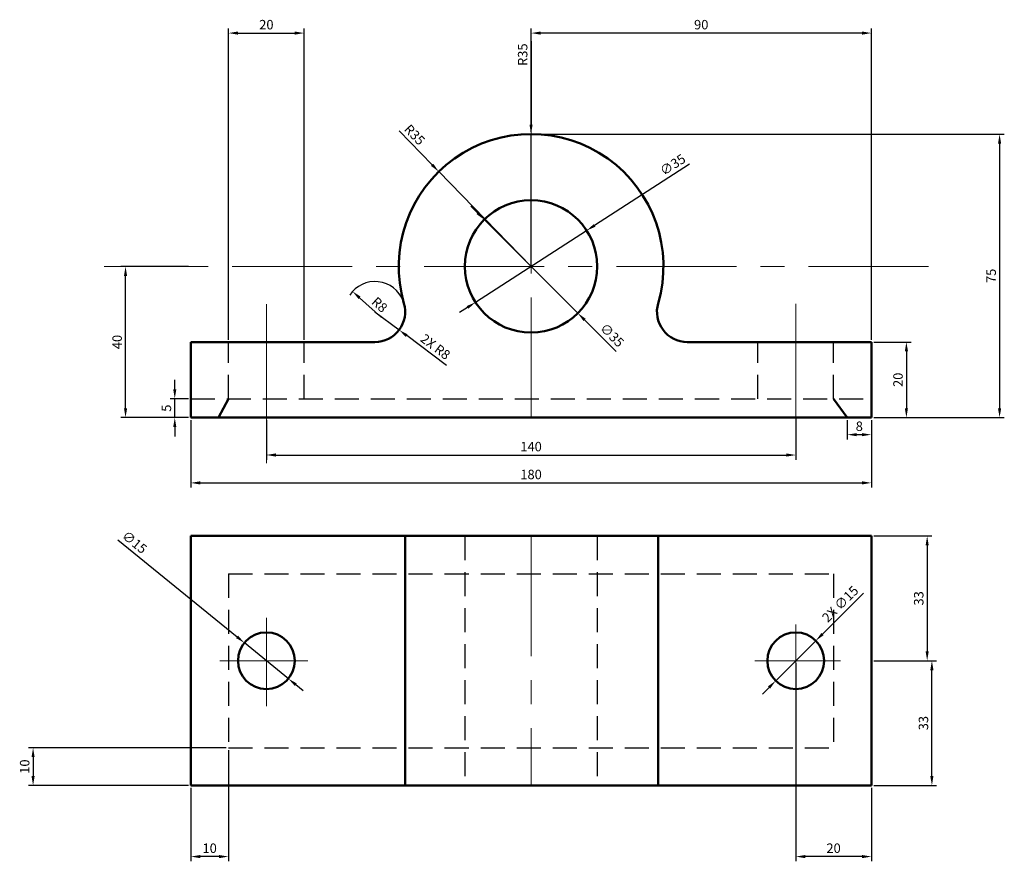
# Model space of a CAD drawing. Units: millimetres. Extents: x 2529 to 2789, y 1399 to 1622.
import ezdxf

# ---------------------------------------------------------------- set-up
doc = ezdxf.new("R2010")
doc.units = ezdxf.units.MM
doc.linetypes.add('CENTER', pattern=[50.8, 31.75, -6.35, 6.35, -6.35])
doc.linetypes.add('HIDDEN', pattern=[9.525, 6.35, -3.175])
for name, color, linetype, lineweight in [('M-CNTR', 1, 'CENTER', 18), ('M-DIMS', 2, 'Continuous', 25), ('M-HIDN', 4, 'HIDDEN', 25), ('M-OUTL', 7, 'Continuous', 50)]:
    doc.layers.add(name, color=color, linetype=linetype, lineweight=lineweight)
doc.styles.get("Standard").update_dxf_attribs({"font": 'arial.ttf'})
doc.dimstyles.new('ISO-25', dxfattribs={"dimtxt": 2.5, "dimasz": 2.5, "dimexe": 1.25, "dimexo": 0.625, "dimtad": 1, "dimtxsty": 'Standard', "dimcen": 2.5, "dimadec": 0, "dimazin": 0, "dimtfac": 1, "dimtmove": 0, "dimatfit": 3, "dimfxl": 1, "dimarcsym": 0})

# ---------------------------------------------------------------- blocks, each defined once
blk = doc.blocks.new('*D1')
at = {"layer": 'Defpoints', "color": 0, "transparency": 16777216}
for p in [(2747.84, 1516.67), (2754.23, 1516.67), (2747.84, 1512.16)]:
    blk.add_point(p, dxfattribs=at)
at = {"layer": 'M-DIMS', "color": 0, "lineweight": -2, "transparency": 16777216}
for p, q in [((2747.84, 1516.04), (2747.84, 1510.91)), ((2754.23, 1516.04), (2754.23, 1510.91)), ((2751.73, 1512.16), (2750.34, 1512.16))]:
    blk.add_line(p, q, dxfattribs=at)
at = {"layer": 'M-DIMS', "color": 0, "transparency": 16777216}
for points in [[(2750.34, 1512.58), (2750.34, 1511.75), (2747.84, 1512.16)], [(2751.73, 1512.58), (2751.73, 1511.75), (2754.23, 1512.16)]]:
    blk.add_solid(points, dxfattribs=at)
at = {"layer": 'M-DIMS', "color": 0, "transparency": 16777216, "insert": (2751.03, 1514.06), "char_height": 2.5, "attachment_point": 5}
blk.add_mtext('8', dxfattribs=at)
blk = doc.blocks.new('*D2')
at = {"layer": 'Defpoints', "color": 0, "transparency": 16777216}
for p in [(2754.23, 1485.36), (2754.23, 1452.36), (2768.98, 1452.36)]:
    blk.add_point(p, dxfattribs=at)
at = {"layer": 'M-DIMS', "color": 0, "lineweight": -2, "transparency": 16777216}
for p, q in [((2754.85, 1485.36), (2770.23, 1485.36)), ((2768.98, 1482.86), (2768.98, 1454.86)), ((2754.85, 1452.36), (2770.23, 1452.36))]:
    blk.add_line(p, q, dxfattribs=at)
at = {"layer": 'M-DIMS', "color": 0, "transparency": 16777216}
for points in [[(2768.56, 1482.86), (2769.39, 1482.86), (2768.98, 1485.36)], [(2768.56, 1454.86), (2769.39, 1454.86), (2768.98, 1452.36)]]:
    blk.add_solid(points, dxfattribs=at)
at = {"layer": 'M-DIMS', "color": 0, "transparency": 16777216, "insert": (2767.07, 1468.86), "char_height": 2.5, "attachment_point": 5, "rotation": 90}
blk.add_mtext('33', dxfattribs=at)
blk = doc.blocks.new('*D3')
at = {"layer": 'Defpoints', "color": 0, "transparency": 16777216}
for p in [(2754.23, 1452.36), (2770.23, 1452.36), (2754.23, 1419.36)]:
    blk.add_point(p, dxfattribs=at)
at = {"layer": 'M-DIMS', "color": 0, "lineweight": -2, "transparency": 16777216}
for p, q in [((2754.85, 1452.36), (2771.48, 1452.36)), ((2770.23, 1421.86), (2770.23, 1449.86)), ((2754.85, 1419.36), (2771.48, 1419.36))]:
    blk.add_line(p, q, dxfattribs=at)
at = {"layer": 'M-DIMS', "color": 0, "transparency": 16777216}
for points in [[(2769.81, 1449.86), (2770.64, 1449.86), (2770.23, 1452.36)], [(2769.81, 1421.86), (2770.64, 1421.86), (2770.23, 1419.36)]]:
    blk.add_solid(points, dxfattribs=at)
at = {"layer": 'M-DIMS', "color": 0, "transparency": 16777216, "insert": (2768.32, 1435.86), "char_height": 2.5, "attachment_point": 5, "rotation": 90}
blk.add_mtext('33', dxfattribs=at)
blk = doc.blocks.new('*D4')
at = {"layer": 'Defpoints', "color": 0, "transparency": 16777216}
for p in [(2588.41, 1457.1), (2600.04, 1447.62)]:
    blk.add_point(p, dxfattribs=at)
at = {"layer": 'M-DIMS', "color": 0, "lineweight": -2, "transparency": 16777216}
for p, q in [((2554.98, 1484.33), (2586.48, 1458.68)), ((2600.04, 1447.62), (2588.41, 1457.1)), ((2601.98, 1446.04), (2603.92, 1444.46))]:
    blk.add_line(p, q, dxfattribs=at)
at = {"layer": 'M-DIMS', "color": 0, "transparency": 16777216}
for points in [[(2586.74, 1459), (2586.21, 1458.35), (2588.41, 1457.1)], [(2602.24, 1446.37), (2601.72, 1445.72), (2600.04, 1447.62)]]:
    blk.add_solid(points, dxfattribs=at)
at = {"layer": 'M-DIMS', "color": 0, "transparency": 16777216, "insert": (2559.16, 1483.47), "char_height": 2.5, "attachment_point": 5, "rotation": 320.8294}
blk.add_mtext('∅15', dxfattribs=at)
blk = doc.blocks.new('*D5')
at = {"layer": 'Defpoints', "color": 0, "transparency": 16777216}
for p in [(2574.23, 1516.67), (2754.23, 1516.67), (2754.23, 1499.41)]:
    blk.add_point(p, dxfattribs=at)
at = {"layer": 'M-DIMS', "color": 0, "lineweight": -2, "transparency": 16777216}
for p, q in [((2574.23, 1516.04), (2574.23, 1498.16)), ((2754.23, 1516.04), (2754.23, 1498.16)), ((2576.73, 1499.41), (2751.73, 1499.41))]:
    blk.add_line(p, q, dxfattribs=at)
at = {"layer": 'M-DIMS', "color": 0, "transparency": 16777216}
for points in [[(2576.73, 1499.83), (2576.73, 1498.99), (2574.23, 1499.41)], [(2751.73, 1499.83), (2751.73, 1498.99), (2754.23, 1499.41)]]:
    blk.add_solid(points, dxfattribs=at)
at = {"layer": 'M-DIMS', "color": 0, "transparency": 16777216, "insert": (2664.23, 1501.31), "char_height": 2.5, "attachment_point": 5}
blk.add_mtext('180', dxfattribs=at)
blk = doc.blocks.new('*D6')
at = {"layer": 'Defpoints', "color": 0, "transparency": 16777216}
for p in [(2594.23, 1516.67), (2734.23, 1517.07), (2734.23, 1506.78)]:
    blk.add_point(p, dxfattribs=at)
at = {"layer": 'M-DIMS', "color": 0, "lineweight": -2, "transparency": 16777216}
for p, q in [((2594.23, 1516.04), (2594.23, 1505.53)), ((2734.23, 1516.44), (2734.23, 1505.53)), ((2596.73, 1506.78), (2731.73, 1506.78))]:
    blk.add_line(p, q, dxfattribs=at)
at = {"layer": 'M-DIMS', "color": 0, "transparency": 16777216}
for points in [[(2596.73, 1507.2), (2596.73, 1506.36), (2594.23, 1506.78)], [(2731.73, 1507.2), (2731.73, 1506.36), (2734.23, 1506.78)]]:
    blk.add_solid(points, dxfattribs=at)
at = {"layer": 'M-DIMS', "color": 0, "transparency": 16777216, "insert": (2664.23, 1508.68), "char_height": 2.5, "attachment_point": 5}
blk.add_mtext('140', dxfattribs=at)
blk = doc.blocks.new('*D7')
at = {"layer": 'Defpoints', "color": 0, "transparency": 16777216}
for p in [(2570.01, 1521.67), (2574.23, 1521.67), (2574.23, 1516.67)]:
    blk.add_point(p, dxfattribs=at)
at = {"layer": 'M-DIMS', "color": 0, "lineweight": -2, "transparency": 16777216}
for p, q in [((2570.01, 1524.17), (2570.01, 1526.67)), ((2573.6, 1521.67), (2568.76, 1521.67)), ((2570.01, 1516.67), (2570.01, 1521.67)), ((2573.6, 1516.67), (2568.76, 1516.67)), ((2570.01, 1514.17), (2570.01, 1511.67))]:
    blk.add_line(p, q, dxfattribs=at)
at = {"layer": 'M-DIMS', "color": 0, "transparency": 16777216}
for points in [[(2569.59, 1524.17), (2570.42, 1524.17), (2570.01, 1521.67)], [(2569.59, 1514.17), (2570.42, 1514.17), (2570.01, 1516.67)]]:
    blk.add_solid(points, dxfattribs=at)
at = {"layer": 'M-DIMS', "color": 0, "transparency": 16777216, "insert": (2568.11, 1519.17), "char_height": 2.5, "attachment_point": 5, "rotation": 90}
blk.add_mtext('5', dxfattribs=at)
blk = doc.blocks.new('*D8')
at = {"layer": 'Defpoints', "color": 0, "transparency": 16777216}
for p in [(2556.98, 1556.67), (2574.23, 1556.67), (2574.23, 1516.67)]:
    blk.add_point(p, dxfattribs=at)
at = {"layer": 'M-DIMS', "color": 0, "lineweight": -2, "transparency": 16777216}
for p, q in [((2573.6, 1556.67), (2555.73, 1556.67)), ((2556.98, 1519.17), (2556.98, 1554.17)), ((2573.6, 1516.67), (2555.73, 1516.67))]:
    blk.add_line(p, q, dxfattribs=at)
at = {"layer": 'M-DIMS', "color": 0, "transparency": 16777216}
for points in [[(2556.57, 1554.17), (2557.4, 1554.17), (2556.98, 1556.67)], [(2556.57, 1519.17), (2557.4, 1519.17), (2556.98, 1516.67)]]:
    blk.add_solid(points, dxfattribs=at)
at = {"layer": 'M-DIMS', "color": 0, "transparency": 16777216, "insert": (2555.08, 1536.67), "char_height": 2.5, "attachment_point": 5, "rotation": 90}
blk.add_mtext('40', dxfattribs=at)
blk = doc.blocks.new('*D9')
at = {"layer": 'Defpoints', "color": 0, "transparency": 16777216}
for p in [(2617.02, 1550.05), (2622.94, 1544.67)]:
    blk.add_point(p, dxfattribs=at)
at = {"layer": 'M-DIMS', "color": 0, "lineweight": -2, "transparency": 16777216}
blk.add_line((2624.63, 1543.13), (2618.87, 1548.37), dxfattribs=at)
blk.add_arc((2622.94, 1544.67), 8, 20.6809, 146.6391, dxfattribs=at)
at = {"layer": 'M-DIMS', "color": 0, "transparency": 16777216}
blk.add_solid([(2619.15, 1548.68), (2618.59, 1548.06), (2617.02, 1550.05)], dxfattribs=at)
at = {"layer": 'M-DIMS', "color": 0, "transparency": 16777216, "insert": (2623.95, 1546.31), "char_height": 2.5, "attachment_point": 5, "rotation": 317.6867}
blk.add_mtext('R8', dxfattribs=at)
blk = doc.blocks.new('*D10')
at = {"layer": 'Defpoints', "color": 0, "transparency": 16777216}
for p in [(2754.23, 1536.67), (2754.23, 1516.67), (2763.49, 1516.67)]:
    blk.add_point(p, dxfattribs=at)
at = {"layer": 'M-DIMS', "color": 0, "lineweight": -2, "transparency": 16777216}
for p, q in [((2754.85, 1536.67), (2764.74, 1536.67)), ((2763.49, 1534.17), (2763.49, 1519.17)), ((2754.85, 1516.67), (2764.74, 1516.67))]:
    blk.add_line(p, q, dxfattribs=at)
at = {"layer": 'M-DIMS', "color": 0, "transparency": 16777216}
for points in [[(2763.07, 1534.17), (2763.91, 1534.17), (2763.49, 1536.67)], [(2763.07, 1519.17), (2763.91, 1519.17), (2763.49, 1516.67)]]:
    blk.add_solid(points, dxfattribs=at)
at = {"layer": 'M-DIMS', "color": 0, "transparency": 16777216, "insert": (2761.59, 1526.67), "char_height": 2.5, "attachment_point": 5, "rotation": 90}
blk.add_mtext('20', dxfattribs=at)
blk = doc.blocks.new('*D11')
at = {"layer": 'Defpoints', "color": 0, "transparency": 16777216}
for p in [(2678.93, 1566.16), (2649.52, 1547.18)]:
    blk.add_point(p, dxfattribs=at)
at = {"layer": 'M-DIMS', "color": 0, "lineweight": -2, "transparency": 16777216}
for p, q in [((2706.1, 1583.69), (2681.03, 1567.51)), ((2649.52, 1547.18), (2678.93, 1566.16)), ((2647.42, 1545.82), (2645.32, 1544.47))]:
    blk.add_line(p, q, dxfattribs=at)
at = {"layer": 'M-DIMS', "color": 0, "transparency": 16777216}
for points in [[(2680.81, 1567.86), (2681.26, 1567.16), (2678.93, 1566.16)], [(2647.2, 1546.17), (2647.65, 1545.47), (2649.52, 1547.18)]]:
    blk.add_solid(points, dxfattribs=at)
at = {"layer": 'M-DIMS', "color": 0, "transparency": 16777216, "insert": (2701.85, 1583.29), "char_height": 2.5, "attachment_point": 5, "rotation": 32.8304}
blk.add_mtext('∅35', dxfattribs=at)
blk = doc.blocks.new('*D12')
at = {"layer": 'Defpoints', "color": 0, "transparency": 16777216}
for p in [(2639.81, 1581.75), (2664.23, 1556.67)]:
    blk.add_point(p, dxfattribs=at)
at = {"layer": 'M-DIMS', "color": 0, "lineweight": -2, "transparency": 16777216}
for p, q in [((2629.31, 1592.54), (2638.07, 1583.54)), ((2664.23, 1556.67), (2639.81, 1581.75))]:
    blk.add_line(p, q, dxfattribs=at)
at = {"layer": 'M-DIMS', "color": 0, "transparency": 16777216}
blk.add_solid([(2638.37, 1583.83), (2637.77, 1583.25), (2639.81, 1581.75)], dxfattribs=at)
at = {"layer": 'M-DIMS', "color": 0, "transparency": 16777216, "insert": (2633.2, 1591.27), "char_height": 2.5, "attachment_point": 5, "rotation": 314.2295}
blk.add_mtext('R35', dxfattribs=at)
blk = doc.blocks.new('MOUNT-HOLE-D15')
blk.add_circle((7.5, 7.5), 7.5)
blk = doc.blocks.new('MOUNT-HOLE-ELEV')
for p, q in [((0, 0), (0, 15)), ((20, 0), (20, 15))]:
    blk.add_line(p, q)
blk = doc.blocks.new('*D15')
at = {"layer": 'Defpoints', "color": 0, "transparency": 16777216}
for p in [(2664.23, 1591.67), (2754.23, 1516.67), (2788.13, 1516.67)]:
    blk.add_point(p, dxfattribs=at)
at = {"layer": 'M-DIMS', "color": 0, "lineweight": -2, "transparency": 16777216}
for p, q in [((2664.85, 1591.67), (2789.38, 1591.67)), ((2788.13, 1589.17), (2788.13, 1519.17)), ((2754.85, 1516.67), (2789.38, 1516.67))]:
    blk.add_line(p, q, dxfattribs=at)
at = {"layer": 'M-DIMS', "color": 0, "transparency": 16777216}
for points in [[(2787.71, 1589.17), (2788.55, 1589.17), (2788.13, 1591.67)], [(2787.71, 1519.17), (2788.55, 1519.17), (2788.13, 1516.67)]]:
    blk.add_solid(points, dxfattribs=at)
at = {"layer": 'M-DIMS', "color": 0, "transparency": 16777216, "insert": (2786.23, 1554.17), "char_height": 2.5, "attachment_point": 5, "rotation": 90}
blk.add_mtext('75', dxfattribs=at)
blk = doc.blocks.new('*D16')
at = {"layer": 'Defpoints', "color": 0, "transparency": 16777216}
for p in [(2734.23, 1452.36), (2754.23, 1419.36), (2734.23, 1400.56)]:
    blk.add_point(p, dxfattribs=at)
at = {"layer": 'M-DIMS', "color": 0, "lineweight": -2, "transparency": 16777216}
for p, q in [((2734.23, 1451.73), (2734.23, 1399.31)), ((2754.23, 1418.73), (2754.23, 1399.31)), ((2751.73, 1400.56), (2736.73, 1400.56))]:
    blk.add_line(p, q, dxfattribs=at)
at = {"layer": 'M-DIMS', "color": 0, "transparency": 16777216}
for points in [[(2736.73, 1400.98), (2736.73, 1400.14), (2734.23, 1400.56)], [(2751.73, 1400.98), (2751.73, 1400.14), (2754.23, 1400.56)]]:
    blk.add_solid(points, dxfattribs=at)
at = {"layer": 'M-DIMS', "color": 0, "transparency": 16777216, "insert": (2744.23, 1402.46), "char_height": 2.5, "attachment_point": 5}
blk.add_mtext('20', dxfattribs=at)
blk = doc.blocks.new('*D17')
at = {"layer": 'Defpoints', "color": 0, "transparency": 16777216}
for p in [(2664.23, 1618.39), (2664.23, 1591.67), (2754.23, 1536.67)]:
    blk.add_point(p, dxfattribs=at)
at = {"layer": 'M-DIMS', "color": 0, "lineweight": -2, "transparency": 16777216}
for p, q in [((2664.23, 1592.29), (2664.23, 1619.64)), ((2754.23, 1537.29), (2754.23, 1619.64)), ((2751.73, 1618.39), (2666.73, 1618.39))]:
    blk.add_line(p, q, dxfattribs=at)
at = {"layer": 'M-DIMS', "color": 0, "transparency": 16777216}
for points in [[(2666.73, 1618.8), (2666.73, 1617.97), (2664.23, 1618.39)], [(2751.73, 1618.8), (2751.73, 1617.97), (2754.23, 1618.39)]]:
    blk.add_solid(points, dxfattribs=at)
at = {"layer": 'M-DIMS', "color": 0, "transparency": 16777216, "insert": (2709.23, 1620.29), "char_height": 2.5, "attachment_point": 5}
blk.add_mtext('90', dxfattribs=at)
blk = doc.blocks.new('*D18')
at = {"layer": 'Defpoints', "color": 0, "transparency": 16777216}
for p in [(2584.23, 1429.36), (2532.53, 1419.36), (2574.23, 1419.36)]:
    blk.add_point(p, dxfattribs=at)
at = {"layer": 'M-DIMS', "color": 0, "lineweight": -2, "transparency": 16777216}
for p, q in [((2583.6, 1429.36), (2531.28, 1429.36)), ((2532.53, 1426.86), (2532.53, 1421.86)), ((2573.6, 1419.36), (2531.28, 1419.36))]:
    blk.add_line(p, q, dxfattribs=at)
at = {"layer": 'M-DIMS', "color": 0, "transparency": 16777216}
for points in [[(2532.12, 1426.86), (2532.95, 1426.86), (2532.53, 1429.36)], [(2532.12, 1421.86), (2532.95, 1421.86), (2532.53, 1419.36)]]:
    blk.add_solid(points, dxfattribs=at)
at = {"layer": 'M-DIMS', "color": 0, "transparency": 16777216, "insert": (2530.63, 1424.36), "char_height": 2.5, "attachment_point": 5, "rotation": 90}
blk.add_mtext('10', dxfattribs=at)
blk = doc.blocks.new('*D19')
at = {"layer": 'Defpoints', "color": 0, "transparency": 16777216}
for p in [(2584.23, 1429.36), (2574.23, 1419.36), (2574.23, 1400.56)]:
    blk.add_point(p, dxfattribs=at)
at = {"layer": 'M-DIMS', "color": 0, "lineweight": -2, "transparency": 16777216}
for p, q in [((2584.23, 1428.73), (2584.23, 1399.31)), ((2574.23, 1418.73), (2574.23, 1399.31)), ((2581.73, 1400.56), (2576.73, 1400.56))]:
    blk.add_line(p, q, dxfattribs=at)
at = {"layer": 'M-DIMS', "color": 0, "transparency": 16777216}
for points in [[(2576.73, 1400.98), (2576.73, 1400.14), (2574.23, 1400.56)], [(2581.73, 1400.98), (2581.73, 1400.14), (2584.23, 1400.56)]]:
    blk.add_solid(points, dxfattribs=at)
at = {"layer": 'M-DIMS', "color": 0, "transparency": 16777216, "insert": (2579.23, 1402.46), "char_height": 2.5, "attachment_point": 5}
blk.add_mtext('10', dxfattribs=at)
blk = doc.blocks.new('*D20')
at = {"layer": 'Defpoints', "color": 0, "transparency": 16777216}
for p in [(2604.23, 1618.39), (2584.23, 1536.67), (2604.23, 1536.67)]:
    blk.add_point(p, dxfattribs=at)
at = {"layer": 'M-DIMS', "color": 0, "lineweight": -2, "transparency": 16777216}
for p, q in [((2584.23, 1537.29), (2584.23, 1619.64)), ((2604.23, 1537.29), (2604.23, 1619.64)), ((2586.73, 1618.39), (2601.73, 1618.39))]:
    blk.add_line(p, q, dxfattribs=at)
at = {"layer": 'M-DIMS', "color": 0, "transparency": 16777216}
for points in [[(2586.73, 1618.8), (2586.73, 1617.97), (2584.23, 1618.39)], [(2601.73, 1618.8), (2601.73, 1617.97), (2604.23, 1618.39)]]:
    blk.add_solid(points, dxfattribs=at)
at = {"layer": 'M-DIMS', "color": 0, "transparency": 16777216, "insert": (2594.23, 1620.29), "char_height": 2.5, "attachment_point": 5}
blk.add_mtext('20', dxfattribs=at)
blk = doc.blocks.new('*D21')
at = {"layer": 'Defpoints', "color": 0, "transparency": 16777216}
for p in [(2664.23, 1591.67), (2664.23, 1556.67)]:
    blk.add_point(p, dxfattribs=at)
at = {"layer": 'M-DIMS', "color": 0, "lineweight": -2, "transparency": 16777216}
for p, q in [((2664.23, 1616.29), (2664.23, 1594.17)), ((2664.23, 1556.67), (2664.23, 1591.67))]:
    blk.add_line(p, q, dxfattribs=at)
at = {"layer": 'M-DIMS', "color": 0, "transparency": 16777216}
blk.add_solid([(2663.81, 1594.17), (2664.64, 1594.17), (2664.23, 1591.67)], dxfattribs=at)
at = {"layer": 'M-DIMS', "color": 0, "transparency": 16777216, "insert": (2662.33, 1612.67), "char_height": 2.5, "attachment_point": 5, "rotation": 89.9999}
blk.add_mtext('R35', dxfattribs=at)
blk = doc.blocks.new('*D22')
at = {"layer": 'Defpoints', "color": 0, "transparency": 16777216}
for p in [(2651.85, 1569.04), (2676.6, 1544.29)]:
    blk.add_point(p, dxfattribs=at)
at = {"layer": 'M-DIMS', "color": 0, "lineweight": -2, "transparency": 16777216}
for p, q in [((2650.09, 1570.81), (2648.32, 1572.58)), ((2651.85, 1569.04), (2676.6, 1544.29)), ((2686.7, 1534.19), (2678.37, 1542.53))]:
    blk.add_line(p, q, dxfattribs=at)
at = {"layer": 'M-DIMS', "color": 0, "transparency": 16777216}
for points in [[(2650.38, 1571.1), (2649.79, 1570.51), (2651.85, 1569.04)], [(2678.66, 1542.82), (2678.08, 1542.23), (2676.6, 1544.29)]]:
    blk.add_solid(points, dxfattribs=at)
at = {"layer": 'M-DIMS', "color": 0, "transparency": 16777216, "insert": (2685.42, 1538.26), "char_height": 2.5, "attachment_point": 5, "rotation": 315.0011}
blk.add_mtext('∅35', dxfattribs=at)
blk = doc.blocks.new('*D23')
at = {"layer": 'Defpoints', "color": 0, "transparency": 16777216}
for p in [(2622.94, 1544.67), (2629.33, 1539.86)]:
    blk.add_point(p, dxfattribs=at)
at = {"layer": 'M-DIMS', "color": 0, "lineweight": -2, "transparency": 16777216}
for p, q in [((2622.94, 1544.67), (2629.33, 1539.86)), ((2641.89, 1530.44), (2631.33, 1538.36))]:
    blk.add_line(p, q, dxfattribs=at)
at = {"layer": 'M-DIMS', "color": 0, "transparency": 16777216}
blk.add_solid([(2631.58, 1538.7), (2631.08, 1538.03), (2629.33, 1539.86)], dxfattribs=at)
at = {"layer": 'M-DIMS', "color": 0, "transparency": 16777216, "insert": (2638.75, 1535.17), "char_height": 2.5, "attachment_point": 5, "rotation": 323.0998}
blk.add_mtext('2X R8', dxfattribs=at)
blk = doc.blocks.new('*D24')
at = {"layer": 'Defpoints', "color": 0, "transparency": 16777216}
for p in [(2739.53, 1457.66), (2728.92, 1447.06)]:
    blk.add_point(p, dxfattribs=at)
at = {"layer": 'M-DIMS', "color": 0, "lineweight": -2, "transparency": 16777216}
for p, q in [((2752.16, 1470.28), (2741.3, 1459.43)), ((2728.92, 1447.06), (2739.53, 1457.66)), ((2727.16, 1445.29), (2725.39, 1443.52))]:
    blk.add_line(p, q, dxfattribs=at)
at = {"layer": 'M-DIMS', "color": 0, "transparency": 16777216}
for points in [[(2741.01, 1459.72), (2741.59, 1459.13), (2739.53, 1457.66)], [(2726.86, 1445.58), (2727.45, 1444.99), (2728.92, 1447.06)]]:
    blk.add_solid(points, dxfattribs=at)
at = {"layer": 'M-DIMS', "color": 0, "transparency": 16777216, "insert": (2746.22, 1467.13), "char_height": 2.5, "attachment_point": 5, "rotation": 44.9926}
blk.add_mtext('2X ∅15', dxfattribs=at)

msp = doc.modelspace()

# ---------------------------------------------------------------- linework, layer by layer
at = {"layer": 'M-CNTR'}
for p, q in [((2664.228, 1516.668), (2664.228, 1599.587)), ((2769.329, 1556.668), (2551.333, 1556.668)), ((2734.228, 1536.668), (2734.228, 1546.804)), ((2734.228, 1546.804), (2734.228, 1517.07)), ((2594.228, 1536.668), (2594.228, 1546.704)), ((2594.228, 1516.668), (2594.228, 1536.668)), ((2734.228, 1516.668), (2734.228, 1536.668)), ((2594.228, 1516.668), (2594.228, 1504.654)), ((2734.228, 1517.07), (2734.228, 1506.358)), ((2664.228, 1485.359), (2664.228, 1419.359)), ((2594.228, 1463.678), (2594.228, 1440.34)), ((2734.228, 1461.943), (2734.228, 1442.847)), ((2581.944, 1452.359), (2605.209, 1452.359)), ((2723.391, 1452.359), (2746.056, 1452.359))]:
    msp.add_line(p, q, dxfattribs=at)
at = {"layer": 'M-HIDN'}
for p, q in [((2574.228, 1521.668), (2754.228, 1521.668)), ((2646.728, 1485.359), (2646.728, 1419.359)), ((2681.728, 1485.359), (2681.728, 1419.359)), ((2584.228, 1475.359), (2744.228, 1475.359)), ((2584.228, 1475.359), (2584.228, 1429.359)), ((2744.228, 1475.359), (2744.228, 1429.359)), ((2584.228, 1429.359), (2744.228, 1429.359))]:
    msp.add_line(p, q, dxfattribs=at)
at = {"layer": 'M-OUTL'}
for p, q in [((2574.228, 1516.668), (2574.228, 1536.668)), ((2574.228, 1536.668), (2622.936, 1536.668)), ((2754.228, 1536.668), (2705.52, 1536.668)), ((2754.228, 1516.668), (2754.228, 1536.668)), ((2584.228, 1521.668), (2581.544, 1516.668)), ((2734.228, 1521.668), (2734.228, 1521.668)), ((2744.228, 1521.668), (2747.841, 1516.668)), ((2574.228, 1516.668), (2754.228, 1516.668)), ((2594.228, 1516.668), (2734.228, 1516.668)), ((2574.228, 1485.359), (2754.228, 1485.359)), ((2574.228, 1485.359), (2574.228, 1419.359)), ((2574.228, 1485.359), (2574.228, 1475.359)), ((2630.936, 1485.359), (2630.936, 1419.359)), ((2697.837, 1485.359), (2697.837, 1419.359)), ((2754.228, 1485.359), (2754.228, 1485.359)), ((2754.228, 1485.359), (2754.228, 1452.359)), ((2754.228, 1452.359), (2754.228, 1419.359)), ((2574.228, 1419.359), (2574.228, 1429.359)), ((2574.228, 1419.359), (2754.228, 1419.359))]:
    msp.add_line(p, q, dxfattribs=at)
msp.add_circle((2664.228, 1556.668), 17.5, dxfattribs=at)
for centre, radius, start, end in [((2664.228, 1556.668), 35, 343.79531, 196.20469), ((2622.936, 1544.668), 8, 270, 16.20469), ((2705.52, 1544.668), 8, 163.79531, 270)]:
    msp.add_arc(centre, radius, start, end, dxfattribs=at)

# ---------------------------------------------------------------- block references
at = {"layer": 'M-HIDN'}
for p in [(2584.228, 1521.668), (2724.228, 1521.668)]:
    msp.add_blockref('MOUNT-HOLE-ELEV', p, dxfattribs=at)
at = {"layer": 'M-OUTL'}
for p in [(2586.728, 1444.859), (2726.728, 1444.859)]:
    msp.add_blockref('MOUNT-HOLE-D15', p, dxfattribs=at)

# ---------------------------------------------------------------- dimensions: what is measured, and where the dimension line sits
at = {"layer": 'M-DIMS'}
for base, p1, p2, override, picture, middle in [((2604.228, 1618.387), (2584.228, 1536.668), (2604.228, 1536.668), {"dimdec": 0, "dimlfac": 1, "dimrnd": 0, "dimzin": 0, "dimdsep": 46, "dimlunit": 2}, '*D20', (2594.228, 1620.289)), ((2664.228, 1618.387), (2754.228, 1536.668), (2664.228, 1591.668), {"dimdec": 0, "dimlfac": 1, "dimrnd": 0, "dimzin": 0, "dimdsep": 46, "dimlunit": 2}, '*D17', (2709.228, 1620.289)), ((2754.228, 1499.41), (2574.228, 1516.668), (2754.228, 1516.668), {"dimclrd": 0, "dimclre": 0, "dimclrt": 0}, '*D5', (2664.228, 1501.312)), ((2734.228, 1506.779), (2594.228, 1516.668), (2734.228, 1517.07), {"dimclrd": 0, "dimclre": 0, "dimclrt": 0}, '*D6', (2664.228, 1508.68)), ((2734.228, 1400.559), (2754.228, 1419.359), (2734.228, 1452.359), {"dimdec": 0, "dimlfac": 1, "dimrnd": 0, "dimzin": 0, "dimdsep": 46, "dimlunit": 2}, '*D16', (2744.228, 1402.461)), ((2574.228, 1400.559), (2584.228, 1429.359), (2574.228, 1419.359), {"dimdec": 0, "dimlfac": 1, "dimrnd": 0, "dimzin": 0, "dimdsep": 46, "dimlunit": 2}, '*D19', (2579.228, 1402.461))]:
    dim = msp.add_linear_dim(base=base, p1=p1, p2=p2, dimstyle='ISO-25', override=override, dxfattribs=at)
    dim.commit()
    dim.dimension.update_dxf_attribs({"geometry": picture, "text_midpoint": middle})
for center, mpoint, override, picture, middle in [((2664.228, 1556.668), (2664.228, 1591.668), {"dimdec": 0, "dimlfac": 1, "dimrnd": 0, "dimzin": 0, "dimdsep": 46, "dimlunit": 2}, '*D21', (2664.228, 1612.668)), ((2664.228, 1556.668), (2639.814, 1581.747), {"dimclrd": 0, "dimclre": 0, "dimclrt": 0}, '*D12', (2631.837, 1589.942)), ((2622.936, 1544.668), (2617.02, 1550.053), {"dimclrd": 0, "dimclre": 0, "dimclrt": 0}, '*D9', (2622.672, 1544.908))]:
    dim = msp.add_radius_dim(center=center, mpoint=mpoint, dimstyle='ISO-25', override=override, dxfattribs=at)
    dim.commit()
    dim.dimension.update_dxf_attribs({"geometry": picture, "text_midpoint": middle, "dimtype": 164})
for base, p1, p2, override, picture, middle in [((2788.129, 1516.668), (2664.228, 1591.668), (2754.228, 1516.668), {"dimdec": 0, "dimlfac": 1, "dimrnd": 0, "dimzin": 0, "dimdsep": 46, "dimlunit": 2}, '*D15', (2786.233, 1554.168)), ((2556.983, 1556.668), (2574.228, 1516.668), (2574.228, 1556.668), {"dimclrd": 0, "dimclre": 0, "dimclrt": 0}, '*D8', (2555.081, 1536.668)), ((2763.491, 1516.668), (2754.228, 1536.668), (2754.228, 1516.668), {"dimclrd": 0, "dimclre": 0, "dimclrt": 0}, '*D10', (2761.589, 1526.668)), ((2570.007, 1521.668), (2574.228, 1516.668), (2574.228, 1521.668), {"dimclrd": 0, "dimclre": 0, "dimclrt": 0}, '*D7', (2568.111, 1519.168)), ((2768.975, 1452.359), (2754.228, 1485.359), (2754.228, 1452.359), {"dimclrd": 0, "dimclre": 0, "dimclrt": 0}, '*D2', (2767.073, 1468.859)), ((2770.225, 1452.359), (2754.228, 1419.359), (2754.228, 1452.359), {"dimclrd": 0, "dimclre": 0, "dimclrt": 0}, '*D3', (2768.323, 1435.859)), ((2532.533, 1419.359), (2584.228, 1429.359), (2574.228, 1419.359), {"dimdec": 0, "dimlfac": 1, "dimrnd": 0, "dimzin": 0, "dimdsep": 46, "dimlunit": 2}, '*D18', (2530.631, 1424.359))]:
    dim = msp.add_linear_dim(base=base, p1=p1, p2=p2, angle=90, dimstyle='ISO-25', override=override, dxfattribs=at)
    dim.commit()
    dim.dimension.update_dxf_attribs({"geometry": picture, "text_midpoint": middle})
for p1, p2, override, picture, middle in [((2649.523, 1547.18), (2678.933, 1566.155), {"dimclrd": 0, "dimclre": 0, "dimclrt": 0}, '*D11', (2702.922, 1581.633)), ((2651.853, 1569.042), (2676.603, 1544.293), {"dimdec": 0, "dimlfac": 1, "dimrnd": 0, "dimzin": 0, "dimdsep": 46, "dimlunit": 2}, '*D22', (2684.027, 1536.869)), ((2600.042, 1447.622), (2588.413, 1457.097), {"dimclrd": 0, "dimclre": 0, "dimclrt": 0}, '*D4', (2557.917, 1481.943))]:
    dim = msp.add_diameter_dim_2p(p1=p1, p2=p2, dimstyle='ISO-25', override=override, dxfattribs=at)
    dim.commit()
    dim.dimension.update_dxf_attribs({"geometry": picture, "text_midpoint": middle, "dimtype": 163})
dim = msp.add_radius_dim(center=(2622.936, 1544.668), mpoint=(2629.334, 1539.864), text='2X <>', dimstyle='ISO-25', override={"dimdec": 0, "dimlfac": 1, "dimrnd": 0, "dimzin": 0, "dimdsep": 46, "dimlunit": 2}, dxfattribs=at)
dim.commit()
dim.dimension.update_dxf_attribs({"geometry": '*D23', "text_midpoint": (2638.752, 1535.17)})
dim = msp.add_linear_dim(base=(2747.841, 1512.163), p1=(2754.228, 1516.668), p2=(2747.841, 1516.668), text='8', dimstyle='ISO-25', override={"dimclrd": 0, "dimclre": 0, "dimclrt": 0}, dxfattribs=at)
dim.commit()
dim.dimension.update_dxf_attribs({"geometry": '*D1', "text_midpoint": (2751.034, 1514.065)})
dim = msp.add_diameter_dim_2p(p1=(2728.924, 1447.057), p2=(2739.532, 1457.662), text='2X <>', dimstyle='ISO-25', override={"dimdec": 0, "dimlfac": 1, "dimrnd": 0, "dimzin": 0, "dimdsep": 46, "dimlunit": 2}, dxfattribs=at)
dim.commit()
dim.dimension.update_dxf_attribs({"geometry": '*D24', "text_midpoint": (2747.612, 1465.74), "dimtype": 163})

doc.saveas('drawing.dxf')
